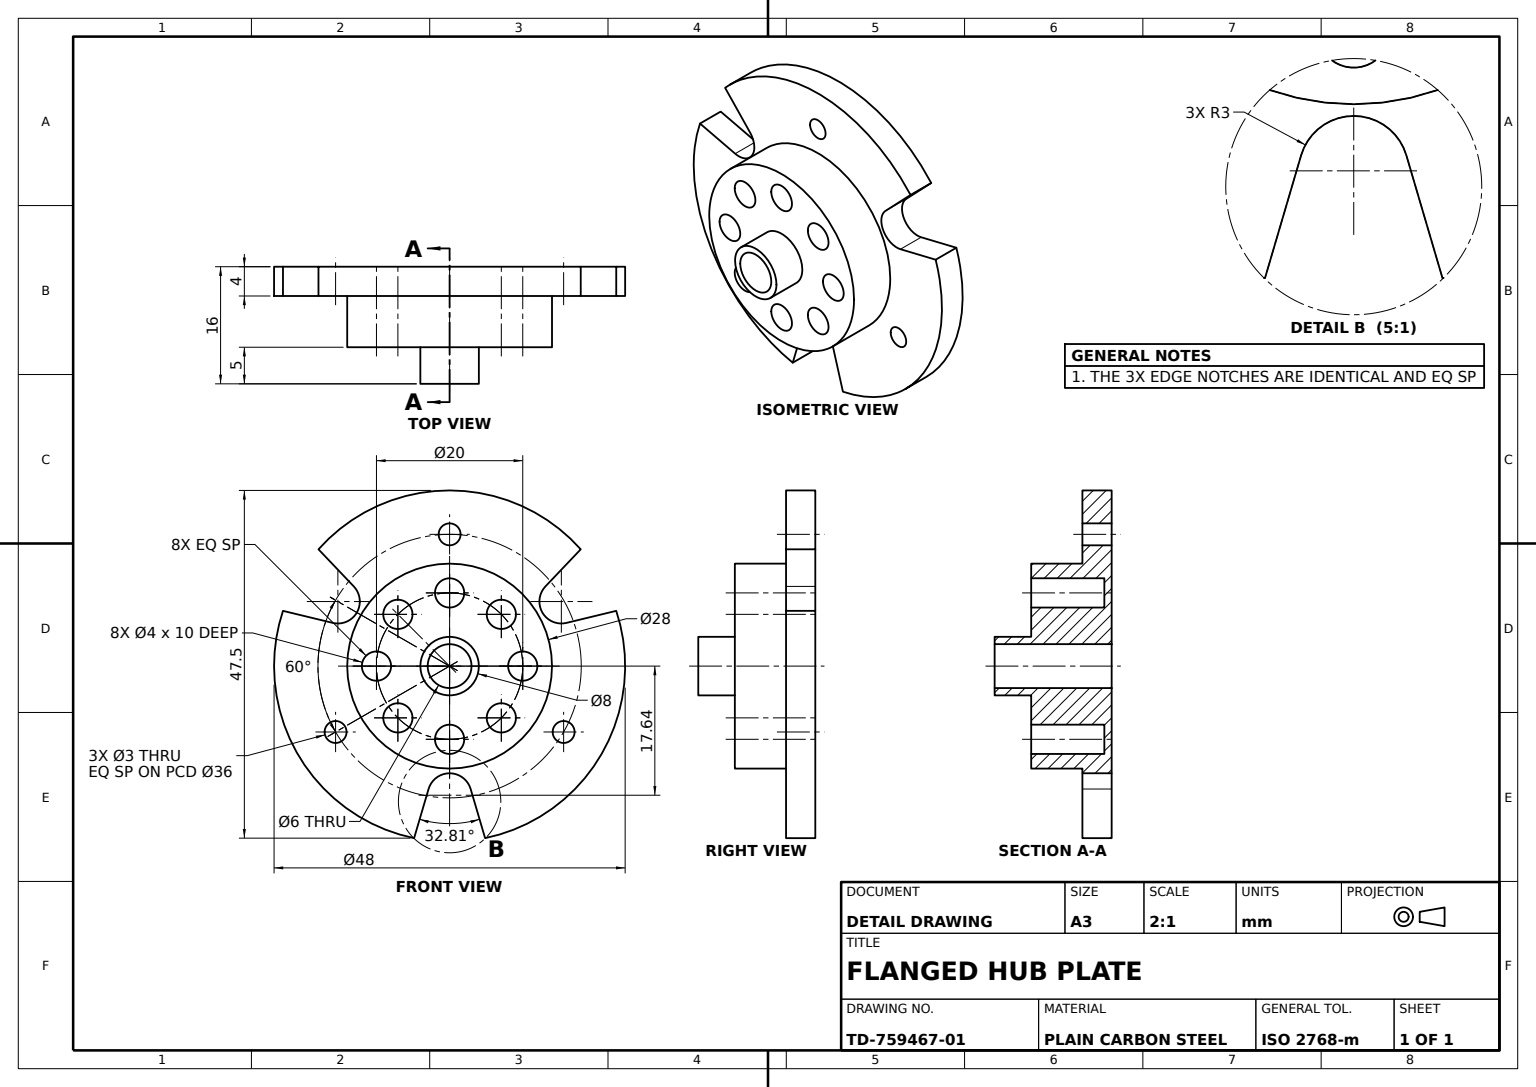
from build123d import *

# Parameters (mm, degrees)
FLANGE_DISC_SKETCH_R    = 24
FLANGE_DISC_48_DEPTH    = 4
HUB_SKETCH_R            = 14
HUB_28_DEPTH            = 7
FLANGE_HOLES_SKETCH_R   = 1.5
FLANGE_HOLES_3X_3_DEPTH = 10
HUB_HOLES_SKETCH_R      = 2
HUB_HOLES_8X_4_DEPTH    = 10
CENTRE_SPIGOT_SKETCH_R  = 4
CENTRE_SPIGOT_8_DEPTH   = 5
BORE_SKETCH_R           = 3
BORE_6_DEPTH            = 30
EDGE_START              = -30
EDGE_NOTCHES_DEPTH      = 30


with BuildPart() as part:
    # Flange Disc Sketch → Flange Disc Ø48 (new body)
    with BuildSketch(Plane.XY):
        Circle(FLANGE_DISC_SKETCH_R)
    extrude(amount=FLANGE_DISC_48_DEPTH)

    # Hub Sketch → Hub Ø28 (add)
    with BuildSketch(Plane.XY.offset(4)):
        Circle(HUB_SKETCH_R)
    extrude(amount=HUB_28_DEPTH)

    # Flange Holes Sketch → Flange Holes 3xØ3 (cut)
    with BuildSketch(Plane.XY.offset(4)):
        with Locations((0, 18)):
            Circle(FLANGE_HOLES_SKETCH_R)
        with Locations((15.588457268, -9)):
            Circle(FLANGE_HOLES_SKETCH_R)
        with Locations((-15.588457268, -9)):
            Circle(FLANGE_HOLES_SKETCH_R)
    extrude(amount=-FLANGE_HOLES_3X_3_DEPTH, mode=Mode.SUBTRACT)

    # Hub Holes Sketch → Hub Holes 8xØ4 (cut)
    with BuildSketch(Plane.XY.offset(11)):
        with Locations((0, 10)):
            Circle(HUB_HOLES_SKETCH_R)
        with Locations((7.071067812, 7.071067812)):
            Circle(HUB_HOLES_SKETCH_R)
        with Locations((10, 0)):
            Circle(HUB_HOLES_SKETCH_R)
        with Locations((7.071067812, -7.071067812)):
            Circle(HUB_HOLES_SKETCH_R)
        with Locations((0, -10)):
            Circle(HUB_HOLES_SKETCH_R)
        with Locations((-7.071067812, -7.071067812)):
            Circle(HUB_HOLES_SKETCH_R)
        with Locations((-10, 0)):
            Circle(HUB_HOLES_SKETCH_R)
        with Locations((-7.071067812, 7.071067812)):
            Circle(HUB_HOLES_SKETCH_R)
    extrude(amount=-HUB_HOLES_8X_4_DEPTH, mode=Mode.SUBTRACT)

    # Centre Spigot Sketch → Centre Spigot Ø8 (add)
    with BuildSketch(Plane.XY.offset(11)):
        Circle(CENTRE_SPIGOT_SKETCH_R)
    extrude(amount=CENTRE_SPIGOT_8_DEPTH)

    # Bore Sketch → Bore Ø6 (cut)
    with BuildSketch(Plane.XY.offset(16)):
        Circle(BORE_SKETCH_R)
    extrude(amount=-BORE_6_DEPTH, mode=Mode.SUBTRACT)

    # Edge Notches Sketch → Edge Notches (cut)
    with BuildSketch(Plane.XY.offset(4).offset(EDGE_START)):
        with BuildLine():
            ThreePointArc((-17.92809871, 15.955665973), (-20.784609691, 12), (-22.782061422, 7.548355939))
            Line((-22.782061422, 7.548355939), (-16.571312466, 6.046586076))
            ThreePointArc((-16.571312466, 6.046586076), (-15.276688123, 8.82), (-13.52215338, 11.327884531))
            Line((-13.52215338, 11.327884531), (-17.92809871, 15.955665973))
        make_face()
        with BuildLine():
            ThreePointArc((-13.52215338, 11.327884531), (-15.276688123, 8.82), (-16.571312466, 6.046586076))
            Line((-16.571312466, 6.046586076), (-15.98177362, 5.904034561))
            ThreePointArc((-15.98177362, 5.904034561), (-12.678611911, 7.32), (-13.103930725, 10.888604672))
            Line((-13.103930725, 10.888604672), (-13.52215338, 11.327884531))
        make_face()
        with BuildLine():
            Line((16.571312466, 6.046586076), (22.782061422, 7.548355939))
            ThreePointArc((22.782061422, 7.548355939), (20.784609691, 12), (17.92809871, 15.955665973))
            Line((17.92809871, 15.955665973), (13.52215338, 11.327884531))
            ThreePointArc((13.52215338, 11.327884531), (15.276688123, 8.82), (16.571312466, 6.046586076))
        make_face()
        with BuildLine():
            ThreePointArc((16.571312466, 6.046586076), (15.276688123, 8.82), (13.52215338, 11.327884531))
            Line((13.52215338, 11.327884531), (13.103930725, 10.888604672))
            ThreePointArc((13.103930725, 10.888604672), (12.678611911, 7.32), (15.98177362, 5.904034561))
            Line((15.98177362, 5.904034561), (16.571312466, 6.046586076))
        make_face()
        with BuildLine():
            Line((-3.049159085, -17.374470607), (-4.853962711, -23.504021911))
            ThreePointArc((-4.853962711, -23.504021911), (0, -24), (4.853962711, -23.504021911))
            Line((4.853962711, -23.504021911), (3.049159085, -17.374470607))
            ThreePointArc((3.049159085, -17.374470607), (0, -17.64), (-3.049159085, -17.374470607))
        make_face()
        with BuildLine():
            Line((-2.877842895, -16.792639233), (-3.049159085, -17.374470607))
            ThreePointArc((-3.049159085, -17.374470607), (0, -17.64), (3.049159085, -17.374470607))
            Line((3.049159085, -17.374470607), (2.877842895, -16.792639233))
            ThreePointArc((2.877842895, -16.792639233), (0, -14.64), (-2.877842895, -16.792639233))
        make_face()
    extrude(amount=EDGE_NOTCHES_DEPTH, mode=Mode.SUBTRACT)


solid = part.part
